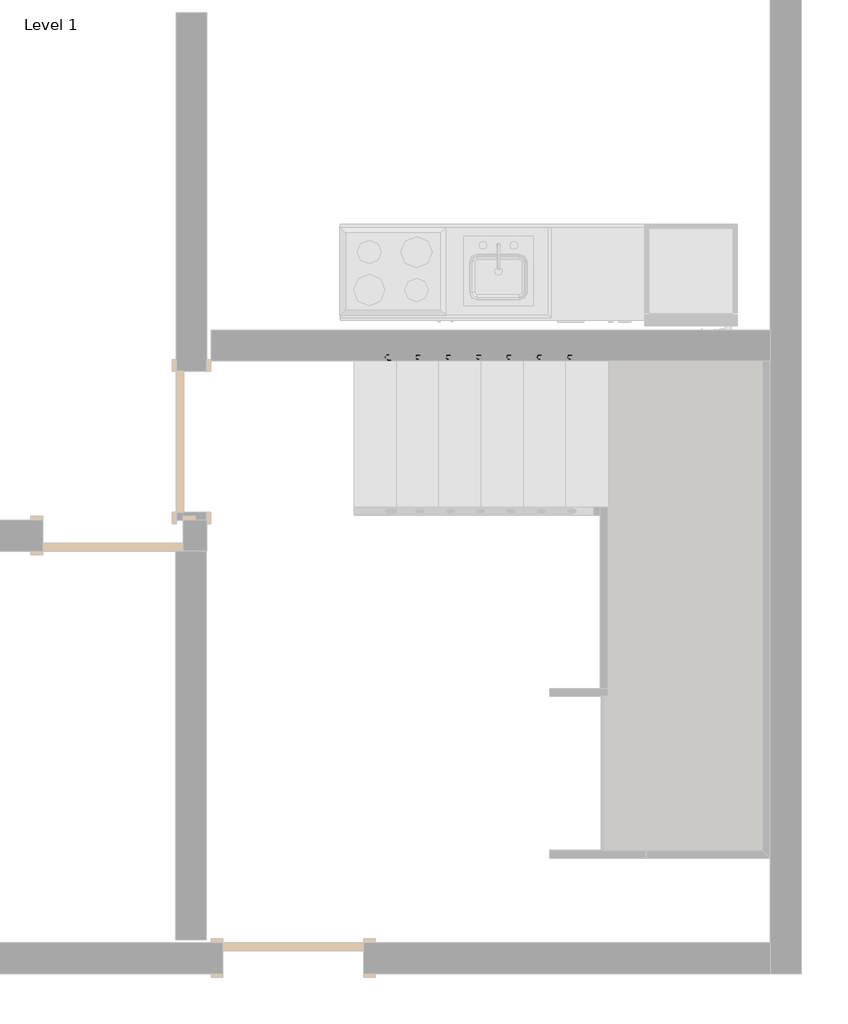
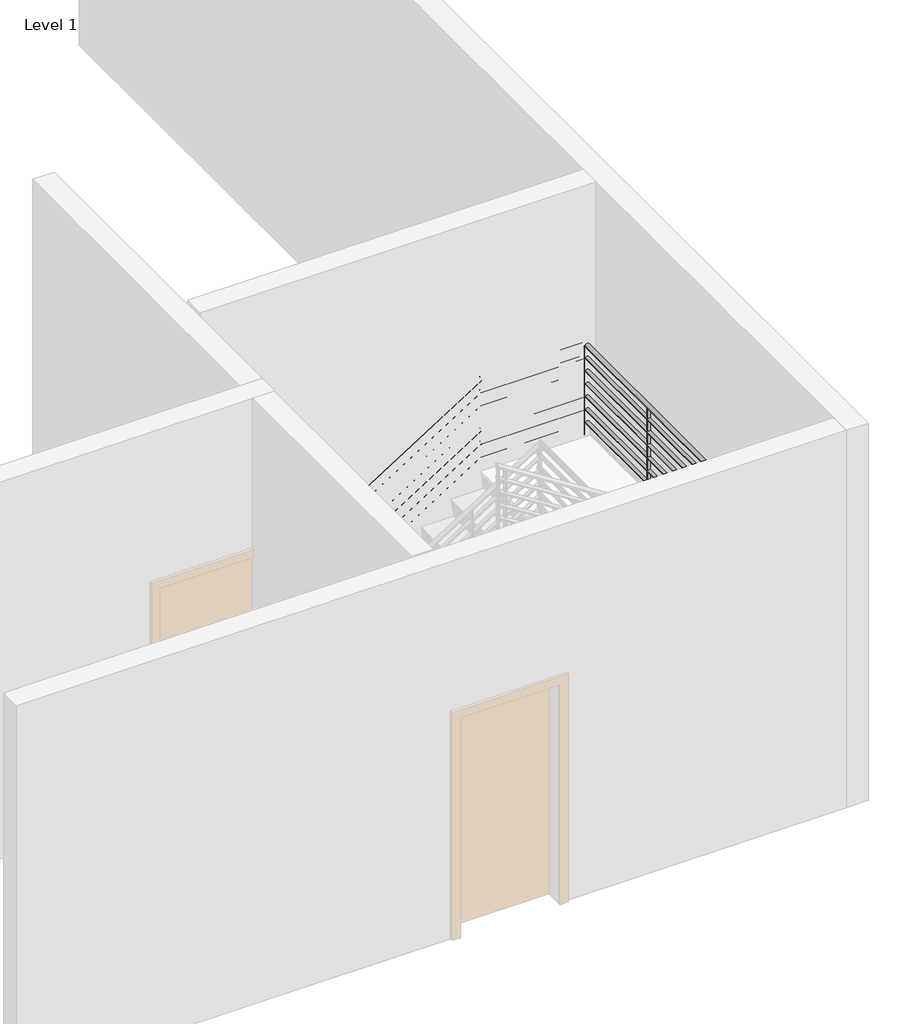
# One storey, part 3 of 4: 1 railing.
"""IFC4 building model written with IfcOpenShell, lengths in millimetres."""

from ifc_helpers import new_model, si_unit, point, frame, frame_2d, origin, place, context, project, spatial, circle_curve, ellipse_curve, trimmed, segment, composite_curve, outline, extrude, element, save
from ifc_brep_helpers import plane_surface, cylinder_surface, advanced_brep

model = new_model("IFC4")

# Units and contexts
model_context = context("Model", 3, world=origin())
ifc_project = project(units=[si_unit("LENGTHUNIT", "METRE", prefix="MILLI")], contexts=[model_context])

# Site, building, storey
site = spatial("IfcSite", under=ifc_project)
building = spatial("IfcBuilding", under=site)
storey = spatial("IfcBuildingStorey", under=building, Name="Level 1", Elevation=0.0)

# Railing
placement = place(None, origin())
element("IfcRailing", 1, ObjectType="900mm Pipe", at=placement, inside=storey, context=model_context, shape_type="SolidModel", body=[
    advanced_brep(
    [(-8739.5726707, 2114.9311514, 1050.2491997), (-8739.5726707, 2154.9311514, 1050.2491997), (-7083.7792177, 2114.9311514, 2097.3913043), (-7083.7792177, 2154.9311514, 2097.3913043), (-6094.9468895, 2154.9311514, 2097.3913043), (-6134.9468895, 2114.9311514, 2097.3913043), (-6134.9468895, -1023.7062768, 2097.3913043), (-6094.9468895, -1063.7062768, 2097.3913043), (-6820.3661237, -1023.7062768, 2097.3913043), (-6820.3661237, -1063.7062768, 2097.3913043), (-8189.5726707, -1023.7062768, 2963.2926779), (-8189.5726707, -1063.7062768, 2963.2926779)],
    [
        (0, 1, ellipse_curve(frame((-8739.5726707, 2134.9311514, 1050.2491997), z_axis=(-1.0, 0.0, 0.0), x_axis=(0.0, 0.0, -1.0)), 23.6638438, 20.0)),
        (1, 0, ellipse_curve(frame((-8739.5726707, 2134.9311514, 1050.2491997), z_axis=(-1.0, 0.0, 0.0), x_axis=(0.0, 0.0, -1.0)), 23.6638438, 20.0)),
        (0, 2),
        (2, 3, ellipse_curve(frame((-7083.7792177, 2134.9311514, 2097.3913043), z_axis=(-0.9605132043335072, 0.0, -0.2782344053149756), x_axis=(0.2782344053149754, 0.0, -0.9605132043335073)), 20.822202, 20.0)),
        (3, 1),
        (3, 2, ellipse_curve(frame((-7083.7792177, 2134.9311514, 2097.3913043), z_axis=(-0.9605132043335072, 0.0, -0.2782344053149756), x_axis=(0.2782344053149754, 0.0, -0.9605132043335073)), 20.822202, 20.0)),
        (4, 5, ellipse_curve(frame((-6114.9468895, 2134.9311514, 2097.3913043), z_axis=(0.7071067811865449, -0.7071067811865501, 0.0), x_axis=(0.7071067811865501, 0.7071067811865449, 0.0)), 28.2842712, 20.0)),
        (5, 6),
        (6, 7, ellipse_curve(frame((-6114.9468895, -1043.7062768, 2097.3913043), z_axis=(0.7071067811865501, 0.7071067811865448, 0.0), x_axis=(-0.7071067811865447, 0.7071067811865503, 0.0)), 28.2842712, 20.0)),
        (7, 4),
        (5, 4, ellipse_curve(frame((-6114.9468895, 2134.9311514, 2097.3913043), z_axis=(0.7071067811865449, -0.7071067811865501, 0.0), x_axis=(0.7071067811865501, 0.7071067811865449, 0.0)), 28.2842712, 20.0)),
        (7, 6, ellipse_curve(frame((-6114.9468895, -1043.7062768, 2097.3913043), z_axis=(0.7071067811865501, 0.7071067811865448, 0.0), x_axis=(-0.7071067811865447, 0.7071067811865503, 0.0)), 28.2842712, 20.0)),
        (6, 8),
        (8, 9, ellipse_curve(frame((-6820.3661237, -1043.7062768, 2097.3913043), z_axis=(0.9605132043335073, 0.0, -0.2782344053149755), x_axis=(0.2782344053149756, 0.0, 0.9605132043335072)), 20.822202, 20.0)),
        (9, 7),
        (9, 8, ellipse_curve(frame((-6820.3661237, -1043.7062768, 2097.3913043), z_axis=(0.9605132043335073, 0.0, -0.2782344053149755), x_axis=(0.2782344053149756, 0.0, 0.9605132043335072)), 20.822202, 20.0)),
        (10, 11, ellipse_curve(frame((-8189.5726707, -1043.7062768, 2963.2926779), z_axis=(-1.0, 0.0, 0.0), x_axis=(0.0, 0.0, -1.0)), 23.6638438, 20.0)),
        (11, 10, ellipse_curve(frame((-8189.5726707, -1043.7062768, 2963.2926779), z_axis=(-1.0, 0.0, 0.0), x_axis=(0.0, 0.0, -1.0)), 23.6638438, 20.0)),
        (8, 10),
        (11, 9),
        (2, 5),
        (4, 3),
    ],
    [
        plane_surface(frame((-8739.5726707, 2134.9311514, 1073.9130435), z_axis=(-1.0, 0.0, 0.0), x_axis=(0.0, 1.0, 0.0))),
        cylinder_surface(frame((-8728.8827579, 2134.9311514, 1057.0096189), z_axis=(-0.8451712313980437, 0.0, -0.5344956404098303), x_axis=(0.0, 1.0, 0.0)), 20.0),
        cylinder_surface(frame((-6114.9468895, 2134.9311514, 2097.3913043), z_axis=(0.0, 1.0, 0.0), x_axis=(1.0, 0.0, 0.0)), 20.0),
        cylinder_surface(frame((-6114.9468895, -1043.7062768, 2097.3913043), z_axis=(1.0, 0.0, 0.0), x_axis=(0.0, -1.0, 0.0)), 20.0),
        plane_surface(frame((-8189.5726707, -1043.7062768, 2986.9565217), z_axis=(-1.0, 0.0, 0.0), x_axis=(0.0, -1.0, 0.0))),
        cylinder_surface(frame((-6825.2625835, -1043.7062768, 2100.4878797), z_axis=(0.8451712313980438, 0.0, -0.5344956404098301), x_axis=(0.0, -1.0, 0.0)), 20.0),
        cylinder_surface(frame((-7089.5726707, 2134.9311514, 2097.3913043), z_axis=(-1.0, 0.0, 0.0), x_axis=(0.0, 1.0, 0.0)), 20.0),
    ],
    [
        (0, [[1, 2]]),
        (1, [[-1, 3, 4, 5]]),
        (1, [[-2, -5, 6, -3]]),
        (2, [[7, 8, 9, 10]]),
        (2, [[11, -10, 12, -8]]),
        (3, [[-9, 13, 14, 15]]),
        (3, [[-12, -15, 16, -13]]),
        (4, [[17, 18]]),
        (5, [[-14, 19, -18, 20]]),
        (5, [[-16, -20, -17, -19]]),
        (6, [[-4, 21, -7, 22]]),
        (6, [[-6, -22, -11, -21]]),
    ],
),
    advanced_brep(
    [(-8739.5726707, 2119.9311514, 931.1651606), (-8739.5726707, 2149.9311514, 931.1651606), (-7085.227581, 2119.9311514, 1977.3913043), (-7085.227581, 2149.9311514, 1977.3913043), (-6129.9468895, 2119.9311514, 1977.3913043), (-6099.9468895, 2149.9311514, 1977.3913043), (-6129.9468895, -1028.7062768, 1977.3913043), (-6099.9468895, -1058.7062768, 1977.3913043), (-6818.9177605, -1028.7062768, 1977.3913043), (-6818.9177605, -1058.7062768, 1977.3913043), (-8189.5726707, -1028.7062768, 2844.2086389), (-8189.5726707, -1058.7062768, 2844.2086389)],
    [
        (0, 1, ellipse_curve(frame((-8739.5726707, 2134.9311514, 931.1651606), z_axis=(-1.0, 0.0, 0.0), x_axis=(0.0, 0.0, -1.0)), 17.7478828, 15.0)),
        (1, 0, ellipse_curve(frame((-8739.5726707, 2134.9311514, 931.1651606), z_axis=(-1.0, 0.0, 0.0), x_axis=(0.0, 0.0, -1.0)), 17.7478828, 15.0)),
        (0, 2),
        (2, 3, ellipse_curve(frame((-7085.227581, 2134.9311514, 1977.3913043), z_axis=(-0.9605132043335072, 0.0, -0.2782344053149755), x_axis=(0.2782344053149752, 0.0, -0.9605132043335075)), 15.6166515, 15.0)),
        (3, 1),
        (3, 2, ellipse_curve(frame((-7085.227581, 2134.9311514, 1977.3913043), z_axis=(-0.9605132043335072, 0.0, -0.2782344053149755), x_axis=(0.2782344053149752, 0.0, -0.9605132043335075)), 15.6166515, 15.0)),
        (2, 4),
        (4, 5, ellipse_curve(frame((-6114.9468895, 2134.9311514, 1977.3913043), z_axis=(-0.7071067811865449, 0.7071067811865501, 0.0), x_axis=(-0.7071067811865501, -0.7071067811865448, 0.0)), 21.2132034, 15.0)),
        (5, 3),
        (5, 4, ellipse_curve(frame((-6114.9468895, 2134.9311514, 1977.3913043), z_axis=(-0.7071067811865449, 0.7071067811865501, 0.0), x_axis=(-0.7071067811865501, -0.7071067811865448, 0.0)), 21.2132034, 15.0)),
        (4, 6),
        (6, 7, ellipse_curve(frame((-6114.9468895, -1043.7062768, 1977.3913043), z_axis=(0.7071067811865501, 0.7071067811865448, 0.0), x_axis=(-0.7071067811865447, 0.7071067811865503, 0.0)), 21.2132034, 15.0)),
        (7, 5),
        (7, 6, ellipse_curve(frame((-6114.9468895, -1043.7062768, 1977.3913043), z_axis=(0.7071067811865501, 0.7071067811865448, 0.0), x_axis=(-0.7071067811865447, 0.7071067811865503, 0.0)), 21.2132034, 15.0)),
        (6, 8),
        (8, 9, ellipse_curve(frame((-6818.9177605, -1043.7062768, 1977.3913043), z_axis=(0.9605132043335072, 0.0, -0.27823440531497556), x_axis=(0.2782344053149759, 0.0, 0.9605132043335071)), 15.6166515, 15.0)),
        (9, 7),
        (9, 8, ellipse_curve(frame((-6818.9177605, -1043.7062768, 1977.3913043), z_axis=(0.9605132043335072, 0.0, -0.27823440531497556), x_axis=(0.2782344053149759, 0.0, 0.9605132043335071)), 15.6166515, 15.0)),
        (10, 11, ellipse_curve(frame((-8189.5726707, -1043.7062768, 2844.2086389), z_axis=(-1.0, 0.0, 0.0), x_axis=(0.0, 0.0, -1.0)), 17.7478828, 15.0)),
        (11, 10, ellipse_curve(frame((-8189.5726707, -1043.7062768, 2844.2086389), z_axis=(-1.0, 0.0, 0.0), x_axis=(0.0, 0.0, -1.0)), 17.7478828, 15.0)),
        (8, 10),
        (11, 9),
    ],
    [
        plane_surface(frame((-8739.5726707, 2134.9311514, 948.9130435), z_axis=(-1.0, 0.0, 0.0), x_axis=(0.0, 1.0, 0.0))),
        cylinder_surface(frame((-8731.5552361, 2134.9311514, 936.235475), z_axis=(-0.8451712313980437, 0.0, -0.5344956404098301), x_axis=(0.0, 1.0, 0.0)), 15.0),
        cylinder_surface(frame((-7089.5726707, 2134.9311514, 1977.3913043), z_axis=(-1.0, 0.0, 0.0), x_axis=(0.0, 1.0, 0.0)), 15.0),
        cylinder_surface(frame((-6114.9468895, 2134.9311514, 1977.3913043), z_axis=(0.0, 1.0, 0.0), x_axis=(1.0, 0.0, 0.0)), 15.0),
        cylinder_surface(frame((-6114.9468895, -1043.7062768, 1977.3913043), z_axis=(1.0, 0.0, 0.0), x_axis=(0.0, -1.0, 0.0)), 15.0),
        plane_surface(frame((-8189.5726707, -1043.7062768, 2861.9565217), z_axis=(-1.0, 0.0, 0.0), x_axis=(0.0, -1.0, 0.0))),
        cylinder_surface(frame((-6822.5901053, -1043.7062768, 1979.7137359), z_axis=(0.8451712313980437, 0.0, -0.5344956404098302), x_axis=(0.0, -1.0, 0.0)), 15.0),
    ],
    [
        (0, [[1, 2]]),
        (1, [[-1, 3, 4, 5]]),
        (1, [[-2, -5, 6, -3]]),
        (2, [[-4, 7, 8, 9]]),
        (2, [[-6, -9, 10, -7]]),
        (3, [[-8, 11, 12, 13]]),
        (3, [[-10, -13, 14, -11]]),
        (4, [[-12, 15, 16, 17]]),
        (4, [[-14, -17, 18, -15]]),
        (5, [[19, 20]]),
        (6, [[-16, 21, -20, 22]]),
        (6, [[-18, -22, -19, -21]]),
    ],
),
    advanced_brep(
    [(-8739.5726707, 2119.9311514, 806.1651606), (-8739.5726707, 2149.9311514, 806.1651606), (-7085.227581, 2119.9311514, 1852.3913043), (-7085.227581, 2149.9311514, 1852.3913043), (-6129.9468895, 2119.9311514, 1852.3913043), (-6099.9468895, 2149.9311514, 1852.3913043), (-6129.9468895, -1028.7062768, 1852.3913043), (-6099.9468895, -1058.7062768, 1852.3913043), (-6818.9177605, -1028.7062768, 1852.3913043), (-6818.9177605, -1058.7062768, 1852.3913043), (-8189.5726707, -1028.7062768, 2719.2086389), (-8189.5726707, -1058.7062768, 2719.2086389)],
    [
        (0, 1, ellipse_curve(frame((-8739.5726707, 2134.9311514, 806.1651606), z_axis=(-1.0, 0.0, 0.0), x_axis=(0.0, 0.0, -1.0)), 17.7478828, 15.0)),
        (1, 0, ellipse_curve(frame((-8739.5726707, 2134.9311514, 806.1651606), z_axis=(-1.0, 0.0, 0.0), x_axis=(0.0, 0.0, -1.0)), 17.7478828, 15.0)),
        (0, 2),
        (2, 3, ellipse_curve(frame((-7085.227581, 2134.9311514, 1852.3913043), z_axis=(-0.9605132043335072, 0.0, -0.2782344053149755), x_axis=(0.2782344053149752, 0.0, -0.9605132043335075)), 15.6166515, 15.0)),
        (3, 1),
        (3, 2, ellipse_curve(frame((-7085.227581, 2134.9311514, 1852.3913043), z_axis=(-0.9605132043335072, 0.0, -0.2782344053149755), x_axis=(0.2782344053149752, 0.0, -0.9605132043335075)), 15.6166515, 15.0)),
        (2, 4),
        (4, 5, ellipse_curve(frame((-6114.9468895, 2134.9311514, 1852.3913043), z_axis=(-0.7071067811865449, 0.7071067811865501, 0.0), x_axis=(-0.7071067811865501, -0.7071067811865448, 0.0)), 21.2132034, 15.0)),
        (5, 3),
        (5, 4, ellipse_curve(frame((-6114.9468895, 2134.9311514, 1852.3913043), z_axis=(-0.7071067811865449, 0.7071067811865501, 0.0), x_axis=(-0.7071067811865501, -0.7071067811865448, 0.0)), 21.2132034, 15.0)),
        (4, 6),
        (6, 7, ellipse_curve(frame((-6114.9468895, -1043.7062768, 1852.3913043), z_axis=(0.7071067811865501, 0.7071067811865448, 0.0), x_axis=(-0.7071067811865447, 0.7071067811865503, 0.0)), 21.2132034, 15.0)),
        (7, 5),
        (7, 6, ellipse_curve(frame((-6114.9468895, -1043.7062768, 1852.3913043), z_axis=(0.7071067811865501, 0.7071067811865448, 0.0), x_axis=(-0.7071067811865447, 0.7071067811865503, 0.0)), 21.2132034, 15.0)),
        (6, 8),
        (8, 9, ellipse_curve(frame((-6818.9177605, -1043.7062768, 1852.3913043), z_axis=(0.9605132043335073, 0.0, -0.2782344053149755), x_axis=(0.2782344053149756, 0.0, 0.9605132043335072)), 15.6166515, 15.0)),
        (9, 7),
        (9, 8, ellipse_curve(frame((-6818.9177605, -1043.7062768, 1852.3913043), z_axis=(0.9605132043335073, 0.0, -0.2782344053149755), x_axis=(0.2782344053149756, 0.0, 0.9605132043335072)), 15.6166515, 15.0)),
        (10, 11, ellipse_curve(frame((-8189.5726707, -1043.7062768, 2719.2086389), z_axis=(-1.0, 0.0, 0.0), x_axis=(0.0, 0.0, -1.0)), 17.7478828, 15.0)),
        (11, 10, ellipse_curve(frame((-8189.5726707, -1043.7062768, 2719.2086389), z_axis=(-1.0, 0.0, 0.0), x_axis=(0.0, 0.0, -1.0)), 17.7478828, 15.0)),
        (8, 10),
        (11, 9),
    ],
    [
        plane_surface(frame((-8739.5726707, 2134.9311514, 823.9130435), z_axis=(-1.0, 0.0, 0.0), x_axis=(0.0, 1.0, 0.0))),
        cylinder_surface(frame((-8731.5552361, 2134.9311514, 811.235475), z_axis=(-0.8451712313980437, 0.0, -0.5344956404098301), x_axis=(0.0, 1.0, 0.0)), 15.0),
        cylinder_surface(frame((-7089.5726707, 2134.9311514, 1852.3913043), z_axis=(-1.0, 0.0, 0.0), x_axis=(0.0, 1.0, 0.0)), 15.0),
        cylinder_surface(frame((-6114.9468895, 2134.9311514, 1852.3913043), z_axis=(0.0, 1.0, 0.0), x_axis=(1.0, 0.0, 0.0)), 15.0),
        cylinder_surface(frame((-6114.9468895, -1043.7062768, 1852.3913043), z_axis=(1.0, 0.0, 0.0), x_axis=(0.0, -1.0, 0.0)), 15.0),
        plane_surface(frame((-8189.5726707, -1043.7062768, 2736.9565217), z_axis=(-1.0, 0.0, 0.0), x_axis=(0.0, -1.0, 0.0))),
        cylinder_surface(frame((-6822.5901053, -1043.7062768, 1854.7137359), z_axis=(0.8451712313980438, 0.0, -0.5344956404098301), x_axis=(0.0, -1.0, 0.0)), 15.0),
    ],
    [
        (0, [[1, 2]]),
        (1, [[-1, 3, 4, 5]]),
        (1, [[-2, -5, 6, -3]]),
        (2, [[-4, 7, 8, 9]]),
        (2, [[-6, -9, 10, -7]]),
        (3, [[-8, 11, 12, 13]]),
        (3, [[-10, -13, 14, -11]]),
        (4, [[-12, 15, 16, 17]]),
        (4, [[-14, -17, 18, -15]]),
        (5, [[19, 20]]),
        (6, [[-16, 21, -20, 22]]),
        (6, [[-18, -22, -19, -21]]),
    ],
),
    advanced_brep(
    [(-8739.5726707, 2119.9311514, 681.1651606), (-8739.5726707, 2149.9311514, 681.1651606), (-7085.227581, 2119.9311514, 1727.3913043), (-7085.227581, 2149.9311514, 1727.3913043), (-6129.9468895, 2119.9311514, 1727.3913043), (-6099.9468895, 2149.9311514, 1727.3913043), (-6129.9468895, -1028.7062768, 1727.3913043), (-6099.9468895, -1058.7062768, 1727.3913043), (-6818.9177605, -1028.7062768, 1727.3913043), (-6818.9177605, -1058.7062768, 1727.3913043), (-8189.5726707, -1028.7062768, 2594.2086389), (-8189.5726707, -1058.7062768, 2594.2086389)],
    [
        (0, 1, ellipse_curve(frame((-8739.5726707, 2134.9311514, 681.1651606), z_axis=(-1.0, 0.0, 0.0), x_axis=(0.0, 0.0, -1.0)), 17.7478828, 15.0)),
        (1, 0, ellipse_curve(frame((-8739.5726707, 2134.9311514, 681.1651606), z_axis=(-1.0, 0.0, 0.0), x_axis=(0.0, 0.0, -1.0)), 17.7478828, 15.0)),
        (0, 2),
        (2, 3, ellipse_curve(frame((-7085.227581, 2134.9311514, 1727.3913043), z_axis=(-0.9605132043335072, 0.0, -0.2782344053149755), x_axis=(0.2782344053149752, 0.0, -0.9605132043335075)), 15.6166515, 15.0)),
        (3, 1),
        (3, 2, ellipse_curve(frame((-7085.227581, 2134.9311514, 1727.3913043), z_axis=(-0.9605132043335072, 0.0, -0.2782344053149755), x_axis=(0.2782344053149752, 0.0, -0.9605132043335075)), 15.6166515, 15.0)),
        (2, 4),
        (4, 5, ellipse_curve(frame((-6114.9468895, 2134.9311514, 1727.3913043), z_axis=(-0.7071067811865449, 0.7071067811865501, 0.0), x_axis=(-0.7071067811865501, -0.7071067811865448, 0.0)), 21.2132034, 15.0)),
        (5, 3),
        (5, 4, ellipse_curve(frame((-6114.9468895, 2134.9311514, 1727.3913043), z_axis=(-0.7071067811865449, 0.7071067811865501, 0.0), x_axis=(-0.7071067811865501, -0.7071067811865448, 0.0)), 21.2132034, 15.0)),
        (4, 6),
        (6, 7, ellipse_curve(frame((-6114.9468895, -1043.7062768, 1727.3913043), z_axis=(0.7071067811865501, 0.7071067811865448, 0.0), x_axis=(-0.7071067811865447, 0.7071067811865503, 0.0)), 21.2132034, 15.0)),
        (7, 5),
        (7, 6, ellipse_curve(frame((-6114.9468895, -1043.7062768, 1727.3913043), z_axis=(0.7071067811865501, 0.7071067811865448, 0.0), x_axis=(-0.7071067811865447, 0.7071067811865503, 0.0)), 21.2132034, 15.0)),
        (6, 8),
        (8, 9, ellipse_curve(frame((-6818.9177605, -1043.7062768, 1727.3913043), z_axis=(0.9605132043335072, 0.0, -0.27823440531497556), x_axis=(0.2782344053149759, 0.0, 0.9605132043335071)), 15.6166515, 15.0)),
        (9, 7),
        (9, 8, ellipse_curve(frame((-6818.9177605, -1043.7062768, 1727.3913043), z_axis=(0.9605132043335072, 0.0, -0.27823440531497556), x_axis=(0.2782344053149759, 0.0, 0.9605132043335071)), 15.6166515, 15.0)),
        (10, 11, ellipse_curve(frame((-8189.5726707, -1043.7062768, 2594.2086389), z_axis=(-1.0, 0.0, 0.0), x_axis=(0.0, 0.0, -1.0)), 17.7478828, 15.0)),
        (11, 10, ellipse_curve(frame((-8189.5726707, -1043.7062768, 2594.2086389), z_axis=(-1.0, 0.0, 0.0), x_axis=(0.0, 0.0, -1.0)), 17.7478828, 15.0)),
        (8, 10),
        (11, 9),
    ],
    [
        plane_surface(frame((-8739.5726707, 2134.9311514, 698.9130435), z_axis=(-1.0, 0.0, 0.0), x_axis=(0.0, 1.0, 0.0))),
        cylinder_surface(frame((-8731.5552361, 2134.9311514, 686.235475), z_axis=(-0.8451712313980437, 0.0, -0.5344956404098301), x_axis=(0.0, 1.0, 0.0)), 15.0),
        cylinder_surface(frame((-7089.5726707, 2134.9311514, 1727.3913043), z_axis=(-1.0, 0.0, 0.0), x_axis=(0.0, 1.0, 0.0)), 15.0),
        cylinder_surface(frame((-6114.9468895, 2134.9311514, 1727.3913043), z_axis=(0.0, 1.0, 0.0), x_axis=(1.0, 0.0, 0.0)), 15.0),
        cylinder_surface(frame((-6114.9468895, -1043.7062768, 1727.3913043), z_axis=(1.0, 0.0, 0.0), x_axis=(0.0, -1.0, 0.0)), 15.0),
        plane_surface(frame((-8189.5726707, -1043.7062768, 2611.9565217), z_axis=(-1.0, 0.0, 0.0), x_axis=(0.0, -1.0, 0.0))),
        cylinder_surface(frame((-6822.5901053, -1043.7062768, 1729.7137359), z_axis=(0.8451712313980437, 0.0, -0.5344956404098302), x_axis=(0.0, -1.0, 0.0)), 15.0),
    ],
    [
        (0, [[1, 2]]),
        (1, [[-1, 3, 4, 5]]),
        (1, [[-2, -5, 6, -3]]),
        (2, [[-4, 7, 8, 9]]),
        (2, [[-6, -9, 10, -7]]),
        (3, [[-8, 11, 12, 13]]),
        (3, [[-10, -13, 14, -11]]),
        (4, [[-12, 15, 16, 17]]),
        (4, [[-14, -17, 18, -15]]),
        (5, [[19, 20]]),
        (6, [[-16, 21, -20, 22]]),
        (6, [[-18, -22, -19, -21]]),
    ],
),
    advanced_brep(
    [(-8739.5726707, 2119.9311514, 556.1651606), (-8739.5726707, 2149.9311514, 556.1651606), (-7085.227581, 2119.9311514, 1602.3913043), (-7085.227581, 2149.9311514, 1602.3913043), (-6129.9468895, 2119.9311514, 1602.3913043), (-6099.9468895, 2149.9311514, 1602.3913043), (-6129.9468895, -1028.7062768, 1602.3913043), (-6099.9468895, -1058.7062768, 1602.3913043), (-6818.9177605, -1028.7062768, 1602.3913043), (-6818.9177605, -1058.7062768, 1602.3913043), (-8189.5726707, -1028.7062768, 2469.2086389), (-8189.5726707, -1058.7062768, 2469.2086389)],
    [
        (0, 1, ellipse_curve(frame((-8739.5726707, 2134.9311514, 556.1651606), z_axis=(-1.0, 0.0, 0.0), x_axis=(0.0, 0.0, -1.0)), 17.7478828, 15.0)),
        (1, 0, ellipse_curve(frame((-8739.5726707, 2134.9311514, 556.1651606), z_axis=(-1.0, 0.0, 0.0), x_axis=(0.0, 0.0, -1.0)), 17.7478828, 15.0)),
        (0, 2),
        (2, 3, ellipse_curve(frame((-7085.227581, 2134.9311514, 1602.3913043), z_axis=(-0.9605132043335072, 0.0, -0.2782344053149755), x_axis=(0.2782344053149752, 0.0, -0.9605132043335075)), 15.6166515, 15.0)),
        (3, 1),
        (3, 2, ellipse_curve(frame((-7085.227581, 2134.9311514, 1602.3913043), z_axis=(-0.9605132043335072, 0.0, -0.2782344053149755), x_axis=(0.2782344053149752, 0.0, -0.9605132043335075)), 15.6166515, 15.0)),
        (2, 4),
        (4, 5, ellipse_curve(frame((-6114.9468895, 2134.9311514, 1602.3913043), z_axis=(-0.7071067811865449, 0.7071067811865501, 0.0), x_axis=(-0.7071067811865501, -0.7071067811865448, 0.0)), 21.2132034, 15.0)),
        (5, 3),
        (5, 4, ellipse_curve(frame((-6114.9468895, 2134.9311514, 1602.3913043), z_axis=(-0.7071067811865449, 0.7071067811865501, 0.0), x_axis=(-0.7071067811865501, -0.7071067811865448, 0.0)), 21.2132034, 15.0)),
        (4, 6),
        (6, 7, ellipse_curve(frame((-6114.9468895, -1043.7062768, 1602.3913043), z_axis=(0.7071067811865501, 0.7071067811865448, 0.0), x_axis=(-0.7071067811865447, 0.7071067811865503, 0.0)), 21.2132034, 15.0)),
        (7, 5),
        (7, 6, ellipse_curve(frame((-6114.9468895, -1043.7062768, 1602.3913043), z_axis=(0.7071067811865501, 0.7071067811865448, 0.0), x_axis=(-0.7071067811865447, 0.7071067811865503, 0.0)), 21.2132034, 15.0)),
        (6, 8),
        (8, 9, ellipse_curve(frame((-6818.9177605, -1043.7062768, 1602.3913043), z_axis=(0.9605132043335073, 0.0, -0.27823440531497573), x_axis=(0.2782344053149754, 0.0, 0.9605132043335073)), 15.6166515, 15.0)),
        (9, 7),
        (9, 8, ellipse_curve(frame((-6818.9177605, -1043.7062768, 1602.3913043), z_axis=(0.9605132043335073, 0.0, -0.27823440531497573), x_axis=(0.2782344053149754, 0.0, 0.9605132043335073)), 15.6166515, 15.0)),
        (10, 11, ellipse_curve(frame((-8189.5726707, -1043.7062768, 2469.2086389), z_axis=(-1.0, 0.0, 0.0), x_axis=(0.0, 0.0, -1.0)), 17.7478828, 15.0)),
        (11, 10, ellipse_curve(frame((-8189.5726707, -1043.7062768, 2469.2086389), z_axis=(-1.0, 0.0, 0.0), x_axis=(0.0, 0.0, -1.0)), 17.7478828, 15.0)),
        (8, 10),
        (11, 9),
    ],
    [
        plane_surface(frame((-8739.5726707, 2134.9311514, 573.9130435), z_axis=(-1.0, 0.0, 0.0), x_axis=(0.0, 1.0, 0.0))),
        cylinder_surface(frame((-8731.5552361, 2134.9311514, 561.235475), z_axis=(-0.8451712313980437, 0.0, -0.5344956404098301), x_axis=(0.0, 1.0, 0.0)), 15.0),
        cylinder_surface(frame((-7089.5726707, 2134.9311514, 1602.3913043), z_axis=(-1.0, 0.0, 0.0), x_axis=(0.0, 1.0, 0.0)), 15.0),
        cylinder_surface(frame((-6114.9468895, 2134.9311514, 1602.3913043), z_axis=(0.0, 1.0, 0.0), x_axis=(1.0, 0.0, 0.0)), 15.0),
        cylinder_surface(frame((-6114.9468895, -1043.7062768, 1602.3913043), z_axis=(1.0, 0.0, 0.0), x_axis=(0.0, -1.0, 0.0)), 15.0),
        plane_surface(frame((-8189.5726707, -1043.7062768, 2486.9565217), z_axis=(-1.0, 0.0, 0.0), x_axis=(0.0, -1.0, 0.0))),
        cylinder_surface(frame((-6822.5901053, -1043.7062768, 1604.7137359), z_axis=(0.8451712313980436, 0.0, -0.5344956404098303), x_axis=(0.0, -1.0, 0.0)), 15.0),
    ],
    [
        (0, [[1, 2]]),
        (1, [[-1, 3, 4, 5]]),
        (1, [[-2, -5, 6, -3]]),
        (2, [[-4, 7, 8, 9]]),
        (2, [[-6, -9, 10, -7]]),
        (3, [[-8, 11, 12, 13]]),
        (3, [[-10, -13, 14, -11]]),
        (4, [[-12, 15, 16, 17]]),
        (4, [[-14, -17, 18, -15]]),
        (5, [[19, 20]]),
        (6, [[-16, 21, -20, 22]]),
        (6, [[-18, -22, -19, -21]]),
    ],
),
    advanced_brep(
    [(-8739.5726707, 2119.9311514, 431.1651606), (-8739.5726707, 2149.9311514, 431.1651606), (-7085.227581, 2119.9311514, 1477.3913043), (-7085.227581, 2149.9311514, 1477.3913043), (-6129.9468895, 2119.9311514, 1477.3913043), (-6099.9468895, 2149.9311514, 1477.3913043), (-6129.9468895, -1028.7062768, 1477.3913043), (-6099.9468895, -1058.7062768, 1477.3913043), (-6818.9177605, -1028.7062768, 1477.3913043), (-6818.9177605, -1058.7062768, 1477.3913043), (-8189.5726707, -1028.7062768, 2344.2086389), (-8189.5726707, -1058.7062768, 2344.2086389)],
    [
        (0, 1, ellipse_curve(frame((-8739.5726707, 2134.9311514, 431.1651606), z_axis=(-1.0, 0.0, 0.0), x_axis=(0.0, 0.0, -1.0)), 17.7478828, 15.0)),
        (1, 0, ellipse_curve(frame((-8739.5726707, 2134.9311514, 431.1651606), z_axis=(-1.0, 0.0, 0.0), x_axis=(0.0, 0.0, -1.0)), 17.7478828, 15.0)),
        (0, 2),
        (2, 3, ellipse_curve(frame((-7085.227581, 2134.9311514, 1477.3913043), z_axis=(-0.9605132043335072, 0.0, -0.2782344053149755), x_axis=(0.2782344053149752, 0.0, -0.9605132043335075)), 15.6166515, 15.0)),
        (3, 1),
        (3, 2, ellipse_curve(frame((-7085.227581, 2134.9311514, 1477.3913043), z_axis=(-0.9605132043335072, 0.0, -0.2782344053149755), x_axis=(0.2782344053149752, 0.0, -0.9605132043335075)), 15.6166515, 15.0)),
        (2, 4),
        (4, 5, ellipse_curve(frame((-6114.9468895, 2134.9311514, 1477.3913043), z_axis=(-0.7071067811865449, 0.7071067811865501, 0.0), x_axis=(-0.7071067811865501, -0.7071067811865448, 0.0)), 21.2132034, 15.0)),
        (5, 3),
        (5, 4, ellipse_curve(frame((-6114.9468895, 2134.9311514, 1477.3913043), z_axis=(-0.7071067811865449, 0.7071067811865501, 0.0), x_axis=(-0.7071067811865501, -0.7071067811865448, 0.0)), 21.2132034, 15.0)),
        (4, 6),
        (6, 7, ellipse_curve(frame((-6114.9468895, -1043.7062768, 1477.3913043), z_axis=(0.7071067811865501, 0.7071067811865448, 0.0), x_axis=(-0.7071067811865447, 0.7071067811865503, 0.0)), 21.2132034, 15.0)),
        (7, 5),
        (7, 6, ellipse_curve(frame((-6114.9468895, -1043.7062768, 1477.3913043), z_axis=(0.7071067811865501, 0.7071067811865448, 0.0), x_axis=(-0.7071067811865447, 0.7071067811865503, 0.0)), 21.2132034, 15.0)),
        (6, 8),
        (8, 9, ellipse_curve(frame((-6818.9177605, -1043.7062768, 1477.3913043), z_axis=(0.9605132043335072, 0.0, -0.27823440531497556), x_axis=(0.2782344053149759, 0.0, 0.9605132043335071)), 15.6166515, 15.0)),
        (9, 7),
        (9, 8, ellipse_curve(frame((-6818.9177605, -1043.7062768, 1477.3913043), z_axis=(0.9605132043335072, 0.0, -0.27823440531497556), x_axis=(0.2782344053149759, 0.0, 0.9605132043335071)), 15.6166515, 15.0)),
        (10, 11, ellipse_curve(frame((-8189.5726707, -1043.7062768, 2344.2086389), z_axis=(-1.0, 0.0, 0.0), x_axis=(0.0, 0.0, -1.0)), 17.7478828, 15.0)),
        (11, 10, ellipse_curve(frame((-8189.5726707, -1043.7062768, 2344.2086389), z_axis=(-1.0, 0.0, 0.0), x_axis=(0.0, 0.0, -1.0)), 17.7478828, 15.0)),
        (8, 10),
        (11, 9),
    ],
    [
        plane_surface(frame((-8739.5726707, 2134.9311514, 448.9130435), z_axis=(-1.0, 0.0, 0.0), x_axis=(0.0, 1.0, 0.0))),
        cylinder_surface(frame((-8731.5552361, 2134.9311514, 436.235475), z_axis=(-0.8451712313980437, 0.0, -0.5344956404098301), x_axis=(0.0, 1.0, 0.0)), 15.0),
        cylinder_surface(frame((-7089.5726707, 2134.9311514, 1477.3913043), z_axis=(-1.0, 0.0, 0.0), x_axis=(0.0, 1.0, 0.0)), 15.0),
        cylinder_surface(frame((-6114.9468895, 2134.9311514, 1477.3913043), z_axis=(0.0, 1.0, 0.0), x_axis=(1.0, 0.0, 0.0)), 15.0),
        cylinder_surface(frame((-6114.9468895, -1043.7062768, 1477.3913043), z_axis=(1.0, 0.0, 0.0), x_axis=(0.0, -1.0, 0.0)), 15.0),
        plane_surface(frame((-8189.5726707, -1043.7062768, 2361.9565217), z_axis=(-1.0, 0.0, 0.0), x_axis=(0.0, -1.0, 0.0))),
        cylinder_surface(frame((-6822.5901053, -1043.7062768, 1479.7137359), z_axis=(0.8451712313980437, 0.0, -0.5344956404098302), x_axis=(0.0, -1.0, 0.0)), 15.0),
    ],
    [
        (0, [[1, 2]]),
        (1, [[-1, 3, 4, 5]]),
        (1, [[-2, -5, 6, -3]]),
        (2, [[-4, 7, 8, 9]]),
        (2, [[-6, -9, 10, -7]]),
        (3, [[-8, 11, 12, 13]]),
        (3, [[-10, -13, 14, -11]]),
        (4, [[-12, 15, 16, 17]]),
        (4, [[-14, -17, 18, -15]]),
        (5, [[19, 20]]),
        (6, [[-16, 21, -20, 22]]),
        (6, [[-18, -22, -19, -21]]),
    ],
),
    advanced_brep(
    [(-8739.5726707, 2119.9311514, 306.1651606), (-8739.5726707, 2149.9311514, 306.1651606), (-7085.227581, 2119.9311514, 1352.3913043), (-7085.227581, 2149.9311514, 1352.3913043), (-6129.9468895, 2119.9311514, 1352.3913043), (-6099.9468895, 2149.9311514, 1352.3913043), (-6129.9468895, -1028.7062768, 1352.3913043), (-6099.9468895, -1058.7062768, 1352.3913043), (-6818.9177605, -1028.7062768, 1352.3913043), (-6818.9177605, -1058.7062768, 1352.3913043), (-8189.5726707, -1028.7062768, 2219.2086389), (-8189.5726707, -1058.7062768, 2219.2086389)],
    [
        (0, 1, ellipse_curve(frame((-8739.5726707, 2134.9311514, 306.1651606), z_axis=(-1.0, 0.0, 0.0), x_axis=(0.0, 0.0, -1.0)), 17.7478828, 15.0)),
        (1, 0, ellipse_curve(frame((-8739.5726707, 2134.9311514, 306.1651606), z_axis=(-1.0, 0.0, 0.0), x_axis=(0.0, 0.0, -1.0)), 17.7478828, 15.0)),
        (0, 2),
        (2, 3, ellipse_curve(frame((-7085.227581, 2134.9311514, 1352.3913043), z_axis=(-0.9605132043335072, 0.0, -0.2782344053149755), x_axis=(0.2782344053149752, 0.0, -0.9605132043335075)), 15.6166515, 15.0)),
        (3, 1),
        (3, 2, ellipse_curve(frame((-7085.227581, 2134.9311514, 1352.3913043), z_axis=(-0.9605132043335072, 0.0, -0.2782344053149755), x_axis=(0.2782344053149752, 0.0, -0.9605132043335075)), 15.6166515, 15.0)),
        (2, 4),
        (4, 5, ellipse_curve(frame((-6114.9468895, 2134.9311514, 1352.3913043), z_axis=(-0.7071067811865449, 0.7071067811865501, 0.0), x_axis=(-0.7071067811865501, -0.7071067811865448, 0.0)), 21.2132034, 15.0)),
        (5, 3),
        (5, 4, ellipse_curve(frame((-6114.9468895, 2134.9311514, 1352.3913043), z_axis=(-0.7071067811865449, 0.7071067811865501, 0.0), x_axis=(-0.7071067811865501, -0.7071067811865448, 0.0)), 21.2132034, 15.0)),
        (4, 6),
        (6, 7, ellipse_curve(frame((-6114.9468895, -1043.7062768, 1352.3913043), z_axis=(0.7071067811865501, 0.7071067811865448, 0.0), x_axis=(-0.7071067811865447, 0.7071067811865503, 0.0)), 21.2132034, 15.0)),
        (7, 5),
        (7, 6, ellipse_curve(frame((-6114.9468895, -1043.7062768, 1352.3913043), z_axis=(0.7071067811865501, 0.7071067811865448, 0.0), x_axis=(-0.7071067811865447, 0.7071067811865503, 0.0)), 21.2132034, 15.0)),
        (6, 8),
        (8, 9, ellipse_curve(frame((-6818.9177605, -1043.7062768, 1352.3913043), z_axis=(0.9605132043335072, 0.0, -0.27823440531497556), x_axis=(0.2782344053149759, 0.0, 0.9605132043335071)), 15.6166515, 15.0)),
        (9, 7),
        (9, 8, ellipse_curve(frame((-6818.9177605, -1043.7062768, 1352.3913043), z_axis=(0.9605132043335072, 0.0, -0.27823440531497556), x_axis=(0.2782344053149759, 0.0, 0.9605132043335071)), 15.6166515, 15.0)),
        (10, 11, ellipse_curve(frame((-8189.5726707, -1043.7062768, 2219.2086389), z_axis=(-1.0, 0.0, 0.0), x_axis=(0.0, 0.0, -1.0)), 17.7478828, 15.0)),
        (11, 10, ellipse_curve(frame((-8189.5726707, -1043.7062768, 2219.2086389), z_axis=(-1.0, 0.0, 0.0), x_axis=(0.0, 0.0, -1.0)), 17.7478828, 15.0)),
        (8, 10),
        (11, 9),
    ],
    [
        plane_surface(frame((-8739.5726707, 2134.9311514, 323.9130435), z_axis=(-1.0, 0.0, 0.0), x_axis=(0.0, 1.0, 0.0))),
        cylinder_surface(frame((-8731.5552361, 2134.9311514, 311.235475), z_axis=(-0.8451712313980437, 0.0, -0.5344956404098301), x_axis=(0.0, 1.0, 0.0)), 15.0),
        cylinder_surface(frame((-7089.5726707, 2134.9311514, 1352.3913043), z_axis=(-1.0, 0.0, 0.0), x_axis=(0.0, 1.0, 0.0)), 15.0),
        cylinder_surface(frame((-6114.9468895, 2134.9311514, 1352.3913043), z_axis=(0.0, 1.0, 0.0), x_axis=(1.0, 0.0, 0.0)), 15.0),
        cylinder_surface(frame((-6114.9468895, -1043.7062768, 1352.3913043), z_axis=(1.0, 0.0, 0.0), x_axis=(0.0, -1.0, 0.0)), 15.0),
        plane_surface(frame((-8189.5726707, -1043.7062768, 2236.9565217), z_axis=(-1.0, 0.0, 0.0), x_axis=(0.0, -1.0, 0.0))),
        cylinder_surface(frame((-6822.5901053, -1043.7062768, 1354.7137359), z_axis=(0.8451712313980437, 0.0, -0.5344956404098302), x_axis=(0.0, -1.0, 0.0)), 15.0),
    ],
    [
        (0, [[1, 2]]),
        (1, [[-1, 3, 4, 5]]),
        (1, [[-2, -5, 6, -3]]),
        (2, [[-4, 7, 8, 9]]),
        (2, [[-6, -9, 10, -7]]),
        (3, [[-8, 11, 12, 13]]),
        (3, [[-10, -13, 14, -11]]),
        (4, [[-12, 15, 16, 17]]),
        (4, [[-14, -17, 18, -15]]),
        (5, [[19, 20]]),
        (6, [[-16, 21, -20, 22]]),
        (6, [[-18, -22, -19, -21]]),
    ],
),
    advanced_brep(
    [(-7814.5726707, -1056.2062768, 2702.474684), (-7814.5726707, -1031.2062768, 2702.474684), (-7814.5726707, -1031.2062768, 1739.1304348), (-7814.5726707, -1056.2062768, 1739.1304348)],
    [
        (0, 1, ellipse_curve(frame((-7814.5726707, -1043.7062768, 2702.474684), z_axis=(-0.5344956404098302, 0.0, -0.8451712313980437), x_axis=(-0.8451712313980437, 0.0, 0.53449564040983)), 14.7899024, 12.5)),
        (1, 2),
        (2, 3, circle_curve(frame((-7814.5726707, -1043.7062768, 1739.1304348), z_axis=(0.0, 0.0, 1.0), x_axis=(0.0, 1.0, 0.0)), 12.5)),
        (3, 0),
        (3, 2, circle_curve(frame((-7814.5726707, -1043.7062768, 1739.1304348), z_axis=(0.0, 0.0, 1.0), x_axis=(0.0, 1.0, 0.0)), 12.5)),
        (1, 0, ellipse_curve(frame((-7814.5726707, -1043.7062768, 2702.474684), z_axis=(-0.5344956404098302, 0.0, -0.8451712313980437), x_axis=(-0.8451712313980437, 0.0, 0.53449564040983)), 14.7899024, 12.5)),
    ],
    [
        cylinder_surface(frame((-7814.5726707, -1043.7062768, 1639.1304348), z_axis=(0.0, 0.0, 1.0), x_axis=(0.0, 1.0, 0.0)), 12.5),
        plane_surface(frame((-7839.5726707, -1018.7062768, 2718.2849606), z_axis=(0.5344956404098302, 0.0, 0.8451712313980437), x_axis=(0.0, -1.0, 0.0))),
        plane_surface(frame((-7789.5726707, -1018.7062768, 1739.1304348), z_axis=(0.0, 0.0, -1.0), x_axis=(0.0, -1.0, 0.0))),
    ],
    [
        (0, [[1, 2, 3, 4]]),
        (0, [[5, -2, 6, -4]]),
        (1, [[-6, -1]]),
        (2, [[-5, -3]]),
    ],
),
    extrude(outline(composite_curve([segment(trimmed(circle_curve(frame_2d((-6114.9468895, -865.0688486)), 12.5), [point((-6127.4468895, -865.0688486))], [point((-6102.4468895, -865.0688486))], False, "CARTESIAN"), True, "CONTINUOUS"), segment(trimmed(circle_curve(frame_2d((-6114.9468895, -865.0688486)), 12.5), [point((-6102.4468895, -865.0688486))], [point((-6127.4468895, -865.0688486))], False, "CARTESIAN"), True, "CONTINUOUS")], self_intersect=False)), frame((0.0, 0.0, 1217.3913043), z_axis=(0.0, 0.0, 1.0), x_axis=(1.0, 0.0, 0.0)), (0.0, 0.0, 1.0), 860.0),
    extrude(outline(composite_curve([segment(trimmed(circle_curve(frame_2d((-6114.9468895, 134.9311514)), 12.5), [point((-6127.4468895, 134.9311514))], [point((-6102.4468895, 134.9311514))], False, "CARTESIAN"), True, "CONTINUOUS"), segment(trimmed(circle_curve(frame_2d((-6114.9468895, 134.9311514)), 12.5), [point((-6102.4468895, 134.9311514))], [point((-6127.4468895, 134.9311514))], False, "CARTESIAN"), True, "CONTINUOUS")], self_intersect=False)), frame((0.0, 0.0, 1217.3913043), z_axis=(0.0, 0.0, 1.0), x_axis=(1.0, 0.0, 0.0)), (0.0, 0.0, 1.0), 860.0),
    extrude(outline(composite_curve([segment(trimmed(circle_curve(frame_2d((-6114.9468895, 1134.9311514)), 12.5), [point((-6127.4468895, 1134.9311514))], [point((-6102.4468895, 1134.9311514))], False, "CARTESIAN"), True, "CONTINUOUS"), segment(trimmed(circle_curve(frame_2d((-6114.9468895, 1134.9311514)), 12.5), [point((-6102.4468895, 1134.9311514))], [point((-6127.4468895, 1134.9311514))], False, "CARTESIAN"), True, "CONTINUOUS")], self_intersect=False)), frame((0.0, 0.0, 1217.3913043), z_axis=(0.0, 0.0, 1.0), x_axis=(1.0, 0.0, 0.0)), (0.0, 0.0, 1.0), 860.0),
    advanced_brep(
    [(-7739.5726707, 2147.4311514, 1658.9964231), (-7739.5726707, 2122.4311514, 1658.9964231), (-7739.5726707, 2122.4311514, 695.6521739), (-7739.5726707, 2147.4311514, 695.6521739)],
    [
        (0, 1, ellipse_curve(frame((-7739.5726707, 2134.9311514, 1658.9964231), z_axis=(0.5344956404098302, 0.0, -0.8451712313980437), x_axis=(0.8451712313980437, 0.0, 0.53449564040983)), 14.7899024, 12.5)),
        (1, 2),
        (2, 3, circle_curve(frame((-7739.5726707, 2134.9311514, 695.6521739), z_axis=(0.0, 0.0, 1.0), x_axis=(0.0, -1.0, 0.0)), 12.5)),
        (3, 0),
        (3, 2, circle_curve(frame((-7739.5726707, 2134.9311514, 695.6521739), z_axis=(0.0, 0.0, 1.0), x_axis=(0.0, -1.0, 0.0)), 12.5)),
        (1, 0, ellipse_curve(frame((-7739.5726707, 2134.9311514, 1658.9964231), z_axis=(0.5344956404098302, 0.0, -0.8451712313980437), x_axis=(0.8451712313980437, 0.0, 0.53449564040983)), 14.7899024, 12.5)),
    ],
    [
        cylinder_surface(frame((-7739.5726707, 2134.9311514, 595.6521739), z_axis=(0.0, 0.0, 1.0), x_axis=(0.0, -1.0, 0.0)), 12.5),
        plane_surface(frame((-7714.5726707, 2109.9311514, 1674.8066998), z_axis=(-0.5344956404098302, 0.0, 0.8451712313980437), x_axis=(0.0, 1.0, 0.0))),
        plane_surface(frame((-7764.5726707, 2109.9311514, 695.6521739), z_axis=(0.0, 0.0, -1.0), x_axis=(0.0, 1.0, 0.0))),
    ],
    [
        (0, [[1, 2, 3, 4]]),
        (0, [[5, -2, 6, -4]]),
        (1, [[-6, -1]]),
        (2, [[-5, -3]]),
    ],
),
    extrude(outline(composite_curve([segment(trimmed(circle_curve(frame_2d((-6814.5726707, -1043.7062768)), 12.5), [point((-6814.5726707, -1031.2062768))], [point((-6814.5726707, -1056.2062768))], False, "CARTESIAN"), True, "CONTINUOUS"), segment(trimmed(circle_curve(frame_2d((-6814.5726707, -1043.7062768)), 12.5), [point((-6814.5726707, -1056.2062768))], [point((-6814.5726707, -1031.2062768))], False, "CARTESIAN"), True, "CONTINUOUS")], self_intersect=False)), frame((0.0, 0.0, 1217.3913043), z_axis=(0.0, 0.0, 1.0), x_axis=(1.0, 0.0, 0.0)), (0.0, 0.0, 1.0), 860.0),
    extrude(outline(composite_curve([segment(trimmed(circle_curve(frame_2d((-6114.9468895, -1043.7062768)), 12.5), [point((-6127.4468895, -1043.7062768))], [point((-6102.4468895, -1043.7062768))], False, "CARTESIAN"), True, "CONTINUOUS"), segment(trimmed(circle_curve(frame_2d((-6114.9468895, -1043.7062768)), 12.5), [point((-6102.4468895, -1043.7062768))], [point((-6127.4468895, -1043.7062768))], False, "CARTESIAN"), True, "CONTINUOUS")], self_intersect=False)), frame((0.0, 0.0, 1217.3913043), z_axis=(0.0, 0.0, 1.0), x_axis=(1.0, 0.0, 0.0)), (0.0, 0.0, 1.0), 860.0),
    extrude(outline(composite_curve([segment(trimmed(circle_curve(frame_2d((-6114.9468895, 2134.9311514)), 12.5), [point((-6114.9468895, 2122.4311514))], [point((-6114.9468895, 2147.4311514))], False, "CARTESIAN"), True, "CONTINUOUS"), segment(trimmed(circle_curve(frame_2d((-6114.9468895, 2134.9311514)), 12.5), [point((-6114.9468895, 2147.4311514))], [point((-6114.9468895, 2122.4311514))], False, "CARTESIAN"), True, "CONTINUOUS")], self_intersect=False)), frame((0.0, 0.0, 1217.3913043), z_axis=(0.0, 0.0, 1.0), x_axis=(1.0, 0.0, 0.0)), (0.0, 0.0, 1.0), 860.0),
    advanced_brep(
    [(-7089.5726707, 2147.4311514, 2070.0636168), (-7089.5726707, 2122.4311514, 2070.0636168), (-7089.5726707, 2122.4311514, 1217.3913043), (-7089.5726707, 2147.4311514, 1217.3913043)],
    [
        (0, 1, ellipse_curve(frame((-7089.5726707, 2134.9311514, 2070.0636168), z_axis=(0.5344956404098286, 0.0, -0.8451712313980447), x_axis=(0.8451712313980447, 0.0, 0.5344956404098286)), 14.7899024, 12.5)),
        (1, 2),
        (2, 3, circle_curve(frame((-7089.5726707, 2134.9311514, 1217.3913043), z_axis=(0.0, 0.0, 1.0), x_axis=(0.0, -1.0, 0.0)), 12.5)),
        (3, 0),
        (3, 2, circle_curve(frame((-7089.5726707, 2134.9311514, 1217.3913043), z_axis=(0.0, 0.0, 1.0), x_axis=(0.0, -1.0, 0.0)), 12.5)),
        (1, 0, ellipse_curve(frame((-7089.5726707, 2134.9311514, 2070.0636168), z_axis=(0.5344956404098286, 0.0, -0.8451712313980447), x_axis=(0.8451712313980447, 0.0, 0.5344956404098286)), 14.7899024, 12.5)),
    ],
    [
        cylinder_surface(frame((-7089.5726707, 2134.9311514, 1117.3913043), z_axis=(0.0, 0.0, 1.0), x_axis=(0.0, -1.0, 0.0)), 12.5),
        plane_surface(frame((-7064.5726707, 2109.9311514, 2085.8738934), z_axis=(-0.5344956404098286, 0.0, 0.8451712313980447), x_axis=(0.0, 1.0, 0.0))),
        plane_surface(frame((-7114.5726707, 2109.9311514, 1217.3913043), z_axis=(0.0, 0.0, -1.0), x_axis=(0.0, 1.0, 0.0))),
    ],
    [
        (0, [[1, 2, 3, 4]]),
        (0, [[5, -2, 6, -4]]),
        (1, [[-6, -1]]),
        (2, [[-5, -3]]),
    ],
),
    advanced_brep(
    [(-8177.0726707, -1056.2062768, 2931.7236958), (-8177.0726707, -1031.2062768, 2931.7236958), (-8177.0726707, -1031.2062768, 1913.0434783), (-8177.0726707, -1056.2062768, 1913.0434783)],
    [
        (0, 1, ellipse_curve(frame((-8177.0726707, -1043.7062768, 2931.7236958), z_axis=(-0.5344956404098319, 0.0, -0.8451712313980426), x_axis=(-0.8451712313980426, 0.0, 0.5344956404098319)), 14.7899024, 12.5)),
        (1, 2),
        (2, 3, circle_curve(frame((-8177.0726707, -1043.7062768, 1913.0434783), z_axis=(0.0, 0.0, 1.0), x_axis=(0.0, 1.0, 0.0)), 12.5)),
        (3, 0),
        (3, 2, circle_curve(frame((-8177.0726707, -1043.7062768, 1913.0434783), z_axis=(0.0, 0.0, 1.0), x_axis=(0.0, 1.0, 0.0)), 12.5)),
        (1, 0, ellipse_curve(frame((-8177.0726707, -1043.7062768, 2931.7236958), z_axis=(-0.5344956404098319, 0.0, -0.8451712313980426), x_axis=(-0.8451712313980426, 0.0, 0.5344956404098319)), 14.7899024, 12.5)),
    ],
    [
        cylinder_surface(frame((-8177.0726707, -1043.7062768, 1813.0434783), z_axis=(0.0, 0.0, 1.0), x_axis=(0.0, 1.0, 0.0)), 12.5),
        plane_surface(frame((-8202.0726707, -1018.7062768, 2947.5339725), z_axis=(0.5344956404098319, 0.0, 0.8451712313980426), x_axis=(0.0, -1.0, 0.0))),
        plane_surface(frame((-8152.0726707, -1018.7062768, 1913.0434783), z_axis=(0.0, 0.0, -1.0), x_axis=(0.0, -1.0, 0.0))),
    ],
    [
        (0, [[1, 2, 3, 4]]),
        (0, [[5, -2, 6, -4]]),
        (1, [[-6, -1]]),
        (2, [[-5, -3]]),
    ],
),
    advanced_brep(
    [(-8727.0726707, 2147.4311514, 1034.4904942), (-8727.0726707, 2122.4311514, 1034.4904942), (-8727.0726707, 2122.4311514, 173.9130435), (-8727.0726707, 2147.4311514, 173.9130435)],
    [
        (0, 1, ellipse_curve(frame((-8727.0726707, 2134.9311514, 1034.4904942), z_axis=(0.5344956404098286, 0.0, -0.8451712313980447), x_axis=(0.8451712313980447, 0.0, 0.5344956404098286)), 14.7899024, 12.5)),
        (1, 2),
        (2, 3, circle_curve(frame((-8727.0726707, 2134.9311514, 173.9130435), z_axis=(0.0, 0.0, 1.0), x_axis=(0.0, -1.0, 0.0)), 12.5)),
        (3, 0),
        (3, 2, circle_curve(frame((-8727.0726707, 2134.9311514, 173.9130435), z_axis=(0.0, 0.0, 1.0), x_axis=(0.0, -1.0, 0.0)), 12.5)),
        (1, 0, ellipse_curve(frame((-8727.0726707, 2134.9311514, 1034.4904942), z_axis=(0.5344956404098286, 0.0, -0.8451712313980447), x_axis=(0.8451712313980447, 0.0, 0.5344956404098286)), 14.7899024, 12.5)),
    ],
    [
        cylinder_surface(frame((-8727.0726707, 2134.9311514, 73.9130435), z_axis=(0.0, 0.0, 1.0), x_axis=(0.0, -1.0, 0.0)), 12.5),
        plane_surface(frame((-8702.0726707, 2109.9311514, 1050.3007709), z_axis=(-0.5344956404098286, 0.0, 0.8451712313980447), x_axis=(0.0, 1.0, 0.0))),
        plane_surface(frame((-8752.0726707, 2109.9311514, 173.9130435), z_axis=(0.0, 0.0, -1.0), x_axis=(0.0, 1.0, 0.0))),
    ],
    [
        (0, [[1, 2, 3, 4]]),
        (0, [[5, -2, 6, -4]]),
        (1, [[-6, -1]]),
        (2, [[-5, -3]]),
    ],
),
])

save(model, "model.ifc")

# Revit data of these elements
# Type "900mm Pipe"
#   built-in parameter 1008612 = 0.019685 (stored number, unit not read)
#   built-in parameter 1008611 = 0.0984252 (stored number, unit not read)
#   built-in parameter 1008609 = 6.56168 (stored number, unit not read)
#   built-in parameter 1008604 = 0.19685 (stored number, unit not read)
#   built-in parameter 1008603 = 0.164042 (stored number, unit not read)
#   Railing Height = 900 mm
#   built-in parameter 1008630 = 2
#   built-in parameter 1008610 = 2
#   built-in parameter 1008605 = 1
#   built-in parameter 1008618 = M_Baluster - Round : 25mm
# Element 1 (IfcRailing, "900mm Pipe")
#   Phase Created = New Construction
